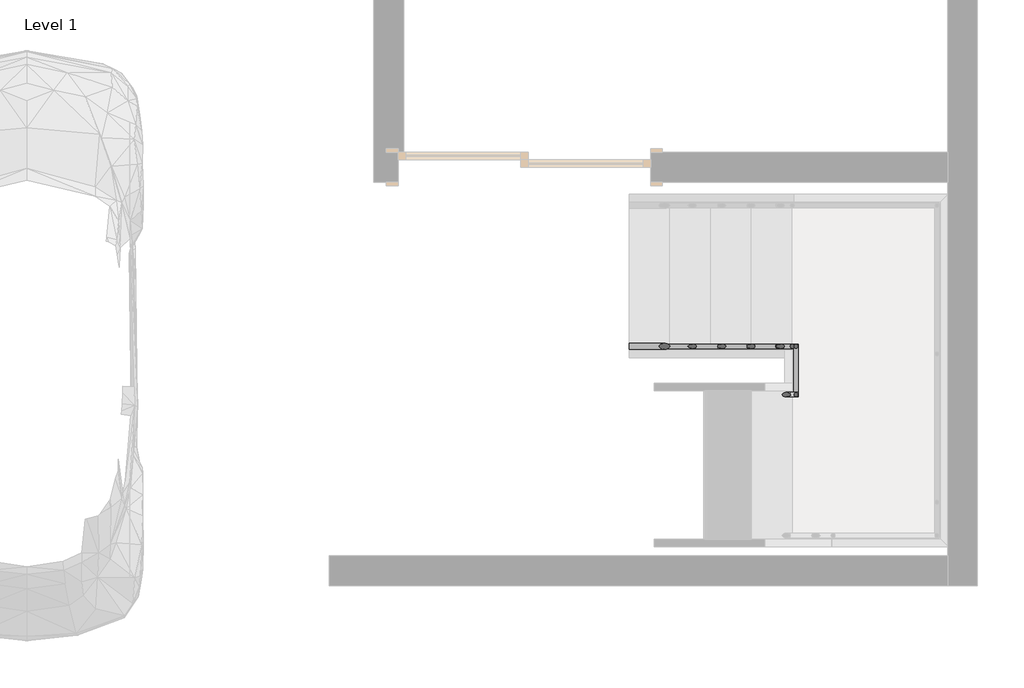
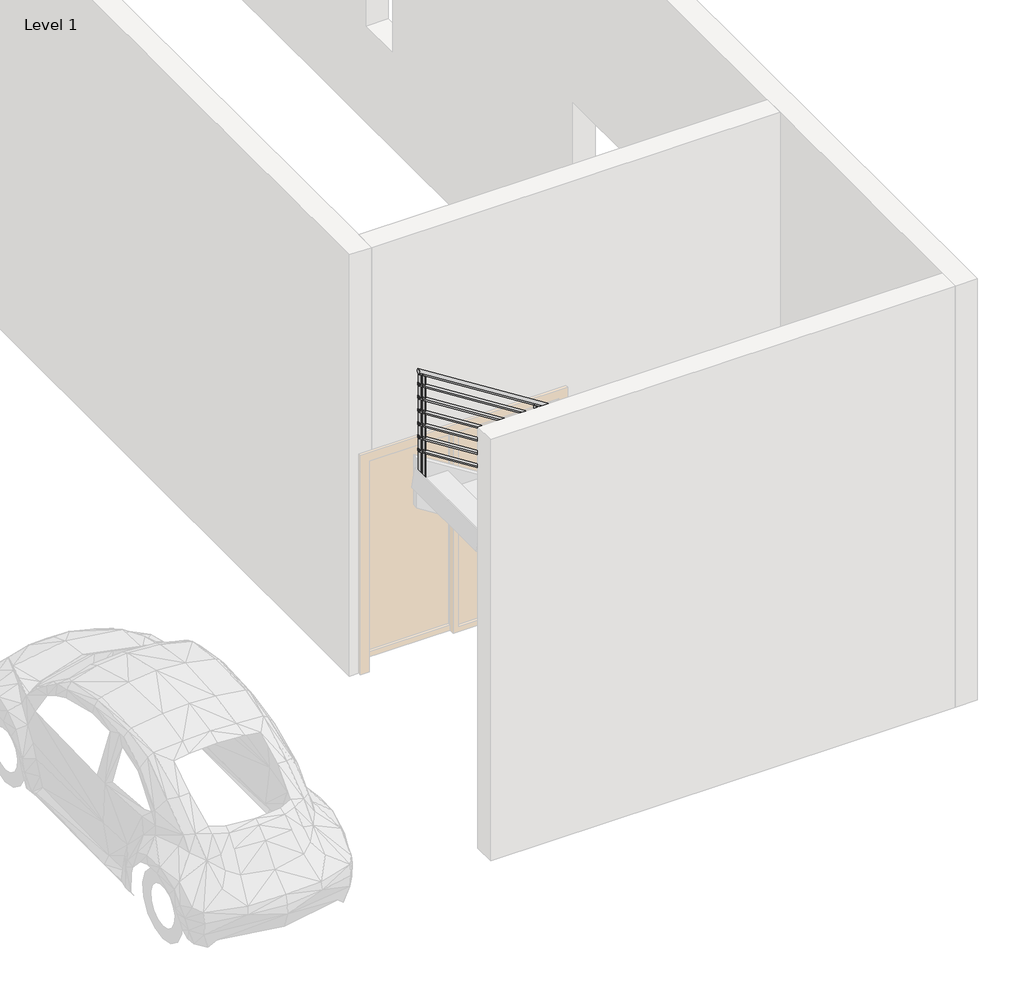
# One storey, part 2 of 4: 1 railing.
"""IFC4 building model written with IfcOpenShell, lengths in millimetres."""

from ifc_helpers import new_model, si_unit, point, frame, frame_2d, origin, place, context, project, spatial, circle_curve, ellipse_curve, trimmed, segment, composite_curve, outline, extrude, element, save
from ifc_brep_helpers import plane_surface, cylinder_surface, advanced_brep

model = new_model("IFC4")

# Units and contexts
model_context = context("Model", 3, world=origin())
ifc_project = project(units=[si_unit("LENGTHUNIT", "METRE", prefix="MILLI")], contexts=[model_context])

# Site, building, storey
site = spatial("IfcSite", under=ifc_project)
building = spatial("IfcBuilding", under=site)
storey = spatial("IfcBuildingStorey", under=building, Name="Level 1", Elevation=0.0)

# Railing
placement = place(None, origin())
element("IfcRailing", 1, ObjectType="900mm Pipe", at=placement, inside=storey, context=model_context, shape_type="SolidModel", body=[
    advanced_brep(
    [(-3791.9701746, -2535.7890637, 1050.2491997), (-3791.9701746, -2495.7890637, 1050.2491997), (-2672.7836865, -2535.7890637, 1758.0351211), (-2638.9768372, -2495.7890637, 1779.4149467)],
    [
        (0, 1, ellipse_curve(frame((-3791.9701746, -2515.7890637, 1050.2491997), z_axis=(-1.0, 0.0, 0.0), x_axis=(0.0, 0.0, -1.0)), 23.6638438, 20.0)),
        (1, 0, ellipse_curve(frame((-3791.9701746, -2515.7890637, 1050.2491997), z_axis=(-1.0, 0.0, 0.0), x_axis=(0.0, 0.0, -1.0)), 23.6638438, 20.0)),
        (2, 3, ellipse_curve(frame((-2655.8802618, -2515.7890637, 1768.7250339), z_axis=(0.5976263089853402, -0.7071067811865487, 0.3779454918484375), x_axis=(-0.5976263089853417, -0.7071067811865465, -0.3779454918484385)), 28.2842712, 20.0)),
        (3, 2, ellipse_curve(frame((-2655.8802618, -2515.7890637, 1768.7250339), z_axis=(0.5976263089853402, -0.7071067811865487, 0.3779454918484375), x_axis=(-0.5976263089853417, -0.7071067811865465, -0.3779454918484385)), 28.2842712, 20.0)),
        (0, 2),
        (3, 1),
    ],
    [
        plane_surface(frame((-3791.9701746, -2515.7890637, 1073.9130435), z_axis=(-1.0, 0.0, 0.0), x_axis=(0.0, 1.0, 0.0))),
        plane_surface(frame((-2666.5701746, -2515.7890637, 1785.6284585), z_axis=(0.5976263089853402, -0.7071067811865487, 0.3779454918484375), x_axis=(0.8017747781070186, 0.5270627453469434, -0.2817127396103774))),
        cylinder_surface(frame((-3781.2802618, -2515.7890637, 1057.0096189), z_axis=(-0.8451712313980431, 0.0, -0.5344956404098311), x_axis=(0.0, 1.0, 0.0)), 20.0),
    ],
    [
        (0, [[1, 2]]),
        (1, [[3, 4]]),
        (2, [[-1, 5, -4, 6]]),
        (2, [[-2, -6, -3, -5]]),
    ],
),
    advanced_brep(
    [(-2686.5701746, -2543.3824011, 1749.5652174), (-2646.5701746, -2509.5755518, 1749.5652174), (-2686.5701746, -2841.5890637, 1749.5652174), (-2646.5701746, -2841.5890637, 1749.5652174)],
    [
        (0, 1, ellipse_curve(frame((-2666.5701746, -2526.4789765, 1749.5652174), z_axis=(-0.5976263089853402, 0.7071067811865487, -0.3779454918484375), x_axis=(0.5976263089853421, 0.7071067811865462, 0.3779454918484387)), 28.2842712, 20.0)),
        (1, 0, ellipse_curve(frame((-2666.5701746, -2526.4789765, 1749.5652174), z_axis=(-0.5976263089853402, 0.7071067811865487, -0.3779454918484375), x_axis=(0.5976263089853421, 0.7071067811865462, 0.3779454918484387)), 28.2842712, 20.0)),
        (2, 3, ellipse_curve(frame((-2666.5701746, -2841.5890637, 1749.5652174), z_axis=(0.0, -0.7071067811865476, 0.7071067811865476), x_axis=(0.0, 0.7071067811865474, 0.7071067811865476)), 28.2842712, 20.0)),
        (3, 2, ellipse_curve(frame((-2666.5701746, -2841.5890637, 1749.5652174), z_axis=(0.0, -0.7071067811865476, 0.7071067811865476), x_axis=(0.0, 0.7071067811865474, 0.7071067811865476)), 28.2842712, 20.0)),
        (0, 2),
        (3, 1),
    ],
    [
        plane_surface(frame((-2666.5701746, -2515.7890637, 1769.5652174), z_axis=(-0.5976263089853402, 0.7071067811865487, -0.3779454918484375), x_axis=(0.8017747781070186, 0.5270627453469434, -0.2817127396103774))),
        plane_surface(frame((-2666.5701746, -2821.5890637, 1769.5652174), z_axis=(0.0, -0.7071067811865476, 0.7071067811865476), x_axis=(1.0, 0.0, 0.0))),
        cylinder_surface(frame((-2666.5701746, -2515.7890637, 1749.5652174), z_axis=(0.0, 1.0, 0.0), x_axis=(1.0, 0.0, 0.0)), 20.0),
    ],
    [
        (0, [[1, 2]]),
        (1, [[3, 4]]),
        (2, [[-1, 5, -4, 6]]),
        (2, [[-2, -6, -3, -5]]),
    ],
),
    advanced_brep(
    [(-2686.5701746, -2841.5890637, 1749.5652174), (-2646.5701746, -2841.5890637, 1749.5652174), (-2686.5701746, -2841.5890637, 1892.7355535), (-2646.5701746, -2841.5890637, 1914.7667984)],
    [
        (0, 1, ellipse_curve(frame((-2666.5701746, -2841.5890637, 1749.5652174), z_axis=(0.0, 0.7071067811865476, -0.7071067811865476), x_axis=(0.0, -0.7071067811865476, -0.7071067811865474)), 28.2842712, 20.0)),
        (1, 0, ellipse_curve(frame((-2666.5701746, -2841.5890637, 1749.5652174), z_axis=(0.0, 0.7071067811865476, -0.7071067811865476), x_axis=(0.0, -0.7071067811865476, -0.7071067811865474)), 28.2842712, 20.0)),
        (2, 3, ellipse_curve(frame((-2666.5701746, -2841.5890637, 1903.751176), z_axis=(-0.4824439654458172, 0.0, 0.8759268349610686), x_axis=(-0.8759268349610686, 0.0, -0.48244396544581725)), 22.8329573, 20.0)),
        (3, 2, ellipse_curve(frame((-2666.5701746, -2841.5890637, 1903.751176), z_axis=(-0.4824439654458172, 0.0, 0.8759268349610686), x_axis=(-0.8759268349610686, 0.0, -0.48244396544581725)), 22.8329573, 20.0)),
        (0, 2),
        (3, 1),
    ],
    [
        plane_surface(frame((-2666.5701746, -2841.5890637, 1749.5652174), z_axis=(0.0, 0.7071067811865476, -0.7071067811865476), x_axis=(1.0, 0.0, 0.0))),
        plane_surface(frame((-2666.5701746, -2841.5890637, 1903.751176), z_axis=(-0.4824439654458172, 0.0, 0.8759268349610686), x_axis=(0.8759268349610686, 0.0, 0.4824439654458172))),
        cylinder_surface(frame((-2666.5701746, -2841.5890637, 1749.5652174), z_axis=(0.0, 0.0, -1.0), x_axis=(1.0, 0.0, 0.0)), 20.0),
    ],
    [
        (0, [[1, 2]]),
        (1, [[3, 4]]),
        (2, [[-1, 5, -4, 6]]),
        (2, [[-2, -6, -3, -5]]),
    ],
),
    advanced_brep(
    [(-2666.5701746, -2821.5890637, 1903.751176), (-2666.5701746, -2861.5890637, 1903.751176), (-5716.9701746, -2821.5890637, 3832.8578953), (-5716.9701746, -2861.5890637, 3832.8578953)],
    [
        (0, 1, ellipse_curve(frame((-2666.5701746, -2841.5890637, 1903.751176), z_axis=(0.4824439654458172, 0.0, -0.8759268349610686), x_axis=(0.8759268349610686, 0.0, 0.48244396544581714)), 22.8329573, 20.0)),
        (1, 0, ellipse_curve(frame((-2666.5701746, -2841.5890637, 1903.751176), z_axis=(0.4824439654458172, 0.0, -0.8759268349610686), x_axis=(0.8759268349610686, 0.0, 0.48244396544581714)), 22.8329573, 20.0)),
        (2, 3, ellipse_curve(frame((-5716.9701746, -2841.5890637, 3832.8578953), z_axis=(-1.0, 0.0, 0.0), x_axis=(0.0, 0.0, -1.0)), 23.6638438, 20.0)),
        (3, 2, ellipse_curve(frame((-5716.9701746, -2841.5890637, 3832.8578953), z_axis=(-1.0, 0.0, 0.0), x_axis=(0.0, 0.0, -1.0)), 23.6638438, 20.0)),
        (0, 2),
        (3, 1),
    ],
    [
        plane_surface(frame((-2646.5701746, -2841.5890637, 1914.7667984), z_axis=(0.4824439654458172, 0.0, -0.8759268349610686), x_axis=(0.8759268349610686, 0.0, 0.4824439654458172))),
        plane_surface(frame((-5716.9701746, -2841.5890637, 3856.5217391), z_axis=(-1.0, 0.0, 0.0), x_axis=(0.0, -1.0, 0.0))),
        cylinder_surface(frame((-2657.2600874, -2841.5890637, 1897.8633738), z_axis=(0.8451712313980437, 0.0, -0.5344956404098302), x_axis=(0.0, -1.0, 0.0)), 20.0),
    ],
    [
        (0, [[1, 2]]),
        (1, [[3, 4]]),
        (2, [[-1, 5, -4, 6]]),
        (2, [[-2, -6, -3, -5]]),
    ],
),
    advanced_brep(
    [(-3791.9701746, -2500.7890637, 931.1651606), (-3791.9701746, -2530.7890637, 931.1651606), (-2687.6250849, -2500.7890637, 1629.5652174), (-2687.6250849, -2530.7890637, 1629.5652174), (-2651.5701746, -2500.7890637, 1629.5652174), (-2681.5701746, -2530.7890637, 1629.5652174), (-2651.5701746, -2826.5890637, 1629.5652174), (-2681.5701746, -2826.5890637, 1629.5652174)],
    [
        (0, 1, ellipse_curve(frame((-3791.9701746, -2515.7890637, 931.1651606), z_axis=(-1.0, 0.0, 0.0), x_axis=(0.0, 0.0, -1.0)), 17.7478828, 15.0)),
        (1, 0, ellipse_curve(frame((-3791.9701746, -2515.7890637, 931.1651606), z_axis=(-1.0, 0.0, 0.0), x_axis=(0.0, 0.0, -1.0)), 17.7478828, 15.0)),
        (0, 2),
        (2, 3, ellipse_curve(frame((-2687.6250849, -2515.7890637, 1629.5652174), z_axis=(-0.9605132043335072, 0.0, -0.2782344053149761), x_axis=(0.27823440531497673, 0.0, -0.960513204333507)), 15.6166515, 15.0)),
        (3, 1),
        (3, 2, ellipse_curve(frame((-2687.6250849, -2515.7890637, 1629.5652174), z_axis=(-0.9605132043335072, 0.0, -0.2782344053149761), x_axis=(0.27823440531497673, 0.0, -0.960513204333507)), 15.6166515, 15.0)),
        (2, 4),
        (4, 5, ellipse_curve(frame((-2666.5701746, -2515.7890637, 1629.5652174), z_axis=(-0.7071067811865461, 0.7071067811865488, 0.0), x_axis=(-0.7071067811865489, -0.707106781186546, 0.0)), 21.2132034, 15.0)),
        (5, 3),
        (5, 4, ellipse_curve(frame((-2666.5701746, -2515.7890637, 1629.5652174), z_axis=(-0.7071067811865461, 0.7071067811865488, 0.0), x_axis=(-0.7071067811865489, -0.707106781186546, 0.0)), 21.2132034, 15.0)),
        (6, 7, circle_curve(frame((-2666.5701746, -2826.5890637, 1629.5652174), z_axis=(0.0, -1.0, 0.0), x_axis=(-1.0, 0.0, 0.0)), 15.0)),
        (7, 6, circle_curve(frame((-2666.5701746, -2826.5890637, 1629.5652174), z_axis=(0.0, -1.0, 0.0), x_axis=(-1.0, 0.0, 0.0)), 15.0)),
        (4, 6),
        (7, 5),
    ],
    [
        plane_surface(frame((-3791.9701746, -2515.7890637, 948.9130435), z_axis=(-1.0, 0.0, 0.0), x_axis=(0.0, 1.0, 0.0))),
        cylinder_surface(frame((-3783.95274, -2515.7890637, 936.235475), z_axis=(-0.8451712313980433, 0.0, -0.534495640409831), x_axis=(0.0, -1.0, 0.0)), 15.0),
        cylinder_surface(frame((-2691.9701746, -2515.7890637, 1629.5652174), z_axis=(-1.0, 0.0, 0.0), x_axis=(0.0, -1.0, 0.0)), 15.0),
        plane_surface(frame((-2666.5701746, -2826.5890637, 1644.5652174), z_axis=(0.0, -1.0, 0.0), x_axis=(0.0, 0.0, -1.0))),
        cylinder_surface(frame((-2666.5701746, -2515.7890637, 1629.5652174), z_axis=(0.0, 1.0, 0.0), x_axis=(-1.0, 0.0, 0.0)), 15.0),
    ],
    [
        (0, [[1, 2]]),
        (1, [[-1, 3, 4, 5]]),
        (1, [[-2, -5, 6, -3]]),
        (2, [[-4, 7, 8, 9]]),
        (2, [[-6, -9, 10, -7]]),
        (3, [[11, 12]]),
        (4, [[-8, 13, -12, 14]]),
        (4, [[-10, -14, -11, -13]]),
    ],
),
    advanced_brep(
    [(-2651.5701746, -2856.5890637, 1775.1809709), (-2651.5701746, -2826.5890637, 1775.1809709), (-5716.9701746, -2856.5890637, 3713.7738563), (-5716.9701746, -2826.5890637, 3713.7738563)],
    [
        (0, 1, ellipse_curve(frame((-2651.5701746, -2841.5890637, 1775.1809709), z_axis=(1.0, 0.0, 0.0), x_axis=(0.0, 0.0, -1.0)), 17.7478828, 15.0)),
        (1, 0, ellipse_curve(frame((-2651.5701746, -2841.5890637, 1775.1809709), z_axis=(1.0, 0.0, 0.0), x_axis=(0.0, 0.0, -1.0)), 17.7478828, 15.0)),
        (2, 3, ellipse_curve(frame((-5716.9701746, -2841.5890637, 3713.7738563), z_axis=(-1.0, 0.0, 0.0), x_axis=(0.0, 0.0, -1.0)), 17.7478828, 15.0)),
        (3, 2, ellipse_curve(frame((-5716.9701746, -2841.5890637, 3713.7738563), z_axis=(-1.0, 0.0, 0.0), x_axis=(0.0, 0.0, -1.0)), 17.7478828, 15.0)),
        (0, 2),
        (3, 1),
    ],
    [
        plane_surface(frame((-2651.5701746, -2841.5890637, 1792.9288538), z_axis=(1.0, 0.0, 0.0), x_axis=(0.0, -1.0, 0.0))),
        plane_surface(frame((-5716.9701746, -2841.5890637, 3731.5217391), z_axis=(-1.0, 0.0, 0.0), x_axis=(0.0, -1.0, 0.0))),
        cylinder_surface(frame((-2659.5876092, -2841.5890637, 1780.2512853), z_axis=(0.8451712313980437, 0.0, -0.5344956404098302), x_axis=(0.0, 1.0, 0.0)), 15.0),
    ],
    [
        (0, [[1, 2]]),
        (1, [[3, 4]]),
        (2, [[-1, 5, -4, 6]]),
        (2, [[-2, -6, -3, -5]]),
    ],
),
    advanced_brep(
    [(-3791.9701746, -2500.7890637, 806.1651606), (-3791.9701746, -2530.7890637, 806.1651606), (-2687.6250849, -2500.7890637, 1504.5652174), (-2687.6250849, -2530.7890637, 1504.5652174), (-2651.5701746, -2500.7890637, 1504.5652174), (-2681.5701746, -2530.7890637, 1504.5652174), (-2651.5701746, -2826.5890637, 1504.5652174), (-2681.5701746, -2826.5890637, 1504.5652174)],
    [
        (0, 1, ellipse_curve(frame((-3791.9701746, -2515.7890637, 806.1651606), z_axis=(-1.0, 0.0, 0.0), x_axis=(0.0, 0.0, -1.0)), 17.7478828, 15.0)),
        (1, 0, ellipse_curve(frame((-3791.9701746, -2515.7890637, 806.1651606), z_axis=(-1.0, 0.0, 0.0), x_axis=(0.0, 0.0, -1.0)), 17.7478828, 15.0)),
        (0, 2),
        (2, 3, ellipse_curve(frame((-2687.6250849, -2515.7890637, 1504.5652174), z_axis=(-0.9605132043335072, 0.0, -0.2782344053149761), x_axis=(0.27823440531497673, 0.0, -0.960513204333507)), 15.6166515, 15.0)),
        (3, 1),
        (3, 2, ellipse_curve(frame((-2687.6250849, -2515.7890637, 1504.5652174), z_axis=(-0.9605132043335072, 0.0, -0.2782344053149761), x_axis=(0.27823440531497673, 0.0, -0.960513204333507)), 15.6166515, 15.0)),
        (2, 4),
        (4, 5, ellipse_curve(frame((-2666.5701746, -2515.7890637, 1504.5652174), z_axis=(-0.7071067811865461, 0.7071067811865488, 0.0), x_axis=(-0.7071067811865489, -0.707106781186546, 0.0)), 21.2132034, 15.0)),
        (5, 3),
        (5, 4, ellipse_curve(frame((-2666.5701746, -2515.7890637, 1504.5652174), z_axis=(-0.7071067811865461, 0.7071067811865488, 0.0), x_axis=(-0.7071067811865489, -0.707106781186546, 0.0)), 21.2132034, 15.0)),
        (6, 7, circle_curve(frame((-2666.5701746, -2826.5890637, 1504.5652174), z_axis=(0.0, -1.0, 0.0), x_axis=(-1.0, 0.0, 0.0)), 15.0)),
        (7, 6, circle_curve(frame((-2666.5701746, -2826.5890637, 1504.5652174), z_axis=(0.0, -1.0, 0.0), x_axis=(-1.0, 0.0, 0.0)), 15.0)),
        (4, 6),
        (7, 5),
    ],
    [
        plane_surface(frame((-3791.9701746, -2515.7890637, 823.9130435), z_axis=(-1.0, 0.0, 0.0), x_axis=(0.0, 1.0, 0.0))),
        cylinder_surface(frame((-3783.95274, -2515.7890637, 811.235475), z_axis=(-0.8451712313980433, 0.0, -0.534495640409831), x_axis=(0.0, -1.0, 0.0)), 15.0),
        cylinder_surface(frame((-2691.9701746, -2515.7890637, 1504.5652174), z_axis=(-1.0, 0.0, 0.0), x_axis=(0.0, -1.0, 0.0)), 15.0),
        plane_surface(frame((-2666.5701746, -2826.5890637, 1519.5652174), z_axis=(0.0, -1.0, 0.0), x_axis=(0.0, 0.0, -1.0))),
        cylinder_surface(frame((-2666.5701746, -2515.7890637, 1504.5652174), z_axis=(0.0, 1.0, 0.0), x_axis=(-1.0, 0.0, 0.0)), 15.0),
    ],
    [
        (0, [[1, 2]]),
        (1, [[-1, 3, 4, 5]]),
        (1, [[-2, -5, 6, -3]]),
        (2, [[-4, 7, 8, 9]]),
        (2, [[-6, -9, 10, -7]]),
        (3, [[11, 12]]),
        (4, [[-8, 13, -12, 14]]),
        (4, [[-10, -14, -11, -13]]),
    ],
),
    advanced_brep(
    [(-2651.5701746, -2856.5890637, 1650.1809709), (-2651.5701746, -2826.5890637, 1650.1809709), (-5716.9701746, -2856.5890637, 3588.7738563), (-5716.9701746, -2826.5890637, 3588.7738563)],
    [
        (0, 1, ellipse_curve(frame((-2651.5701746, -2841.5890637, 1650.1809709), z_axis=(1.0, 0.0, 0.0), x_axis=(0.0, 0.0, -1.0)), 17.7478828, 15.0)),
        (1, 0, ellipse_curve(frame((-2651.5701746, -2841.5890637, 1650.1809709), z_axis=(1.0, 0.0, 0.0), x_axis=(0.0, 0.0, -1.0)), 17.7478828, 15.0)),
        (2, 3, ellipse_curve(frame((-5716.9701746, -2841.5890637, 3588.7738563), z_axis=(-1.0, 0.0, 0.0), x_axis=(0.0, 0.0, -1.0)), 17.7478828, 15.0)),
        (3, 2, ellipse_curve(frame((-5716.9701746, -2841.5890637, 3588.7738563), z_axis=(-1.0, 0.0, 0.0), x_axis=(0.0, 0.0, -1.0)), 17.7478828, 15.0)),
        (0, 2),
        (3, 1),
    ],
    [
        plane_surface(frame((-2651.5701746, -2841.5890637, 1667.9288538), z_axis=(1.0, 0.0, 0.0), x_axis=(0.0, -1.0, 0.0))),
        plane_surface(frame((-5716.9701746, -2841.5890637, 3606.5217391), z_axis=(-1.0, 0.0, 0.0), x_axis=(0.0, -1.0, 0.0))),
        cylinder_surface(frame((-2659.5876092, -2841.5890637, 1655.2512853), z_axis=(0.8451712313980437, 0.0, -0.5344956404098302), x_axis=(0.0, 1.0, 0.0)), 15.0),
    ],
    [
        (0, [[1, 2]]),
        (1, [[3, 4]]),
        (2, [[-1, 5, -4, 6]]),
        (2, [[-2, -6, -3, -5]]),
    ],
),
    advanced_brep(
    [(-3791.9701746, -2500.7890637, 681.1651606), (-3791.9701746, -2530.7890637, 681.1651606), (-2687.6250849, -2500.7890637, 1379.5652174), (-2687.6250849, -2530.7890637, 1379.5652174), (-2651.5701746, -2500.7890637, 1379.5652174), (-2681.5701746, -2530.7890637, 1379.5652174), (-2651.5701746, -2826.5890637, 1379.5652174), (-2681.5701746, -2826.5890637, 1379.5652174)],
    [
        (0, 1, ellipse_curve(frame((-3791.9701746, -2515.7890637, 681.1651606), z_axis=(-1.0, 0.0, 0.0), x_axis=(0.0, 0.0, -1.0)), 17.7478828, 15.0)),
        (1, 0, ellipse_curve(frame((-3791.9701746, -2515.7890637, 681.1651606), z_axis=(-1.0, 0.0, 0.0), x_axis=(0.0, 0.0, -1.0)), 17.7478828, 15.0)),
        (0, 2),
        (2, 3, ellipse_curve(frame((-2687.6250849, -2515.7890637, 1379.5652174), z_axis=(-0.9605132043335072, 0.0, -0.2782344053149761), x_axis=(0.27823440531497673, 0.0, -0.960513204333507)), 15.6166515, 15.0)),
        (3, 1),
        (3, 2, ellipse_curve(frame((-2687.6250849, -2515.7890637, 1379.5652174), z_axis=(-0.9605132043335072, 0.0, -0.2782344053149761), x_axis=(0.27823440531497673, 0.0, -0.960513204333507)), 15.6166515, 15.0)),
        (2, 4),
        (4, 5, ellipse_curve(frame((-2666.5701746, -2515.7890637, 1379.5652174), z_axis=(-0.7071067811865461, 0.7071067811865488, 0.0), x_axis=(-0.7071067811865489, -0.707106781186546, 0.0)), 21.2132034, 15.0)),
        (5, 3),
        (5, 4, ellipse_curve(frame((-2666.5701746, -2515.7890637, 1379.5652174), z_axis=(-0.7071067811865461, 0.7071067811865488, 0.0), x_axis=(-0.7071067811865489, -0.707106781186546, 0.0)), 21.2132034, 15.0)),
        (6, 7, circle_curve(frame((-2666.5701746, -2826.5890637, 1379.5652174), z_axis=(0.0, -1.0, 0.0), x_axis=(-1.0, 0.0, 0.0)), 15.0)),
        (7, 6, circle_curve(frame((-2666.5701746, -2826.5890637, 1379.5652174), z_axis=(0.0, -1.0, 0.0), x_axis=(-1.0, 0.0, 0.0)), 15.0)),
        (4, 6),
        (7, 5),
    ],
    [
        plane_surface(frame((-3791.9701746, -2515.7890637, 698.9130435), z_axis=(-1.0, 0.0, 0.0), x_axis=(0.0, 1.0, 0.0))),
        cylinder_surface(frame((-3783.95274, -2515.7890637, 686.235475), z_axis=(-0.8451712313980433, 0.0, -0.534495640409831), x_axis=(0.0, -1.0, 0.0)), 15.0),
        cylinder_surface(frame((-2691.9701746, -2515.7890637, 1379.5652174), z_axis=(-1.0, 0.0, 0.0), x_axis=(0.0, -1.0, 0.0)), 15.0),
        plane_surface(frame((-2666.5701746, -2826.5890637, 1394.5652174), z_axis=(0.0, -1.0, 0.0), x_axis=(0.0, 0.0, -1.0))),
        cylinder_surface(frame((-2666.5701746, -2515.7890637, 1379.5652174), z_axis=(0.0, 1.0, 0.0), x_axis=(-1.0, 0.0, 0.0)), 15.0),
    ],
    [
        (0, [[1, 2]]),
        (1, [[-1, 3, 4, 5]]),
        (1, [[-2, -5, 6, -3]]),
        (2, [[-4, 7, 8, 9]]),
        (2, [[-6, -9, 10, -7]]),
        (3, [[11, 12]]),
        (4, [[-8, 13, -12, 14]]),
        (4, [[-10, -14, -11, -13]]),
    ],
),
    advanced_brep(
    [(-2651.5701746, -2856.5890637, 1525.1809709), (-2651.5701746, -2826.5890637, 1525.1809709), (-5716.9701746, -2856.5890637, 3463.7738563), (-5716.9701746, -2826.5890637, 3463.7738563)],
    [
        (0, 1, ellipse_curve(frame((-2651.5701746, -2841.5890637, 1525.1809709), z_axis=(1.0, 0.0, 0.0), x_axis=(0.0, 0.0, -1.0)), 17.7478828, 15.0)),
        (1, 0, ellipse_curve(frame((-2651.5701746, -2841.5890637, 1525.1809709), z_axis=(1.0, 0.0, 0.0), x_axis=(0.0, 0.0, -1.0)), 17.7478828, 15.0)),
        (2, 3, ellipse_curve(frame((-5716.9701746, -2841.5890637, 3463.7738563), z_axis=(-1.0, 0.0, 0.0), x_axis=(0.0, 0.0, -1.0)), 17.7478828, 15.0)),
        (3, 2, ellipse_curve(frame((-5716.9701746, -2841.5890637, 3463.7738563), z_axis=(-1.0, 0.0, 0.0), x_axis=(0.0, 0.0, -1.0)), 17.7478828, 15.0)),
        (0, 2),
        (3, 1),
    ],
    [
        plane_surface(frame((-2651.5701746, -2841.5890637, 1542.9288538), z_axis=(1.0, 0.0, 0.0), x_axis=(0.0, -1.0, 0.0))),
        plane_surface(frame((-5716.9701746, -2841.5890637, 3481.5217391), z_axis=(-1.0, 0.0, 0.0), x_axis=(0.0, -1.0, 0.0))),
        cylinder_surface(frame((-2659.5876092, -2841.5890637, 1530.2512853), z_axis=(0.8451712313980437, 0.0, -0.5344956404098301), x_axis=(0.0, 1.0, 0.0)), 15.0),
    ],
    [
        (0, [[1, 2]]),
        (1, [[3, 4]]),
        (2, [[-1, 5, -4, 6]]),
        (2, [[-2, -6, -3, -5]]),
    ],
),
    advanced_brep(
    [(-3791.9701746, -2500.7890637, 556.1651606), (-3791.9701746, -2530.7890637, 556.1651606), (-2687.6250849, -2500.7890637, 1254.5652174), (-2687.6250849, -2530.7890637, 1254.5652174), (-2651.5701746, -2500.7890637, 1254.5652174), (-2681.5701746, -2530.7890637, 1254.5652174), (-2651.5701746, -2826.5890637, 1254.5652174), (-2681.5701746, -2826.5890637, 1254.5652174)],
    [
        (0, 1, ellipse_curve(frame((-3791.9701746, -2515.7890637, 556.1651606), z_axis=(-1.0, 0.0, 0.0), x_axis=(0.0, 0.0, -1.0)), 17.7478828, 15.0)),
        (1, 0, ellipse_curve(frame((-3791.9701746, -2515.7890637, 556.1651606), z_axis=(-1.0, 0.0, 0.0), x_axis=(0.0, 0.0, -1.0)), 17.7478828, 15.0)),
        (0, 2),
        (2, 3, ellipse_curve(frame((-2687.6250849, -2515.7890637, 1254.5652174), z_axis=(-0.9605132043335072, 0.0, -0.2782344053149761), x_axis=(0.27823440531497673, 0.0, -0.960513204333507)), 15.6166515, 15.0)),
        (3, 1),
        (3, 2, ellipse_curve(frame((-2687.6250849, -2515.7890637, 1254.5652174), z_axis=(-0.9605132043335072, 0.0, -0.2782344053149761), x_axis=(0.27823440531497673, 0.0, -0.960513204333507)), 15.6166515, 15.0)),
        (2, 4),
        (4, 5, ellipse_curve(frame((-2666.5701746, -2515.7890637, 1254.5652174), z_axis=(-0.7071067811865461, 0.7071067811865488, 0.0), x_axis=(-0.7071067811865489, -0.707106781186546, 0.0)), 21.2132034, 15.0)),
        (5, 3),
        (5, 4, ellipse_curve(frame((-2666.5701746, -2515.7890637, 1254.5652174), z_axis=(-0.7071067811865461, 0.7071067811865488, 0.0), x_axis=(-0.7071067811865489, -0.707106781186546, 0.0)), 21.2132034, 15.0)),
        (6, 7, circle_curve(frame((-2666.5701746, -2826.5890637, 1254.5652174), z_axis=(0.0, -1.0, 0.0), x_axis=(-1.0, 0.0, 0.0)), 15.0)),
        (7, 6, circle_curve(frame((-2666.5701746, -2826.5890637, 1254.5652174), z_axis=(0.0, -1.0, 0.0), x_axis=(-1.0, 0.0, 0.0)), 15.0)),
        (4, 6),
        (7, 5),
    ],
    [
        plane_surface(frame((-3791.9701746, -2515.7890637, 573.9130435), z_axis=(-1.0, 0.0, 0.0), x_axis=(0.0, 1.0, 0.0))),
        cylinder_surface(frame((-3783.95274, -2515.7890637, 561.235475), z_axis=(-0.8451712313980433, 0.0, -0.534495640409831), x_axis=(0.0, -1.0, 0.0)), 15.0),
        cylinder_surface(frame((-2691.9701746, -2515.7890637, 1254.5652174), z_axis=(-1.0, 0.0, 0.0), x_axis=(0.0, -1.0, 0.0)), 15.0),
        plane_surface(frame((-2666.5701746, -2826.5890637, 1269.5652174), z_axis=(0.0, -1.0, 0.0), x_axis=(0.0, 0.0, -1.0))),
        cylinder_surface(frame((-2666.5701746, -2515.7890637, 1254.5652174), z_axis=(0.0, 1.0, 0.0), x_axis=(-1.0, 0.0, 0.0)), 15.0),
    ],
    [
        (0, [[1, 2]]),
        (1, [[-1, 3, 4, 5]]),
        (1, [[-2, -5, 6, -3]]),
        (2, [[-4, 7, 8, 9]]),
        (2, [[-6, -9, 10, -7]]),
        (3, [[11, 12]]),
        (4, [[-8, 13, -12, 14]]),
        (4, [[-10, -14, -11, -13]]),
    ],
),
    advanced_brep(
    [(-2651.5701746, -2856.5890637, 1400.1809709), (-2651.5701746, -2826.5890637, 1400.1809709), (-5716.9701746, -2856.5890637, 3338.7738563), (-5716.9701746, -2826.5890637, 3338.7738563)],
    [
        (0, 1, ellipse_curve(frame((-2651.5701746, -2841.5890637, 1400.1809709), z_axis=(1.0, 0.0, 0.0), x_axis=(0.0, 0.0, -1.0)), 17.7478828, 15.0)),
        (1, 0, ellipse_curve(frame((-2651.5701746, -2841.5890637, 1400.1809709), z_axis=(1.0, 0.0, 0.0), x_axis=(0.0, 0.0, -1.0)), 17.7478828, 15.0)),
        (2, 3, ellipse_curve(frame((-5716.9701746, -2841.5890637, 3338.7738563), z_axis=(-1.0, 0.0, 0.0), x_axis=(0.0, 0.0, -1.0)), 17.7478828, 15.0)),
        (3, 2, ellipse_curve(frame((-5716.9701746, -2841.5890637, 3338.7738563), z_axis=(-1.0, 0.0, 0.0), x_axis=(0.0, 0.0, -1.0)), 17.7478828, 15.0)),
        (0, 2),
        (3, 1),
    ],
    [
        plane_surface(frame((-2651.5701746, -2841.5890637, 1417.9288538), z_axis=(1.0, 0.0, 0.0), x_axis=(0.0, -1.0, 0.0))),
        plane_surface(frame((-5716.9701746, -2841.5890637, 3356.5217391), z_axis=(-1.0, 0.0, 0.0), x_axis=(0.0, -1.0, 0.0))),
        cylinder_surface(frame((-2659.5876092, -2841.5890637, 1405.2512853), z_axis=(0.8451712313980437, 0.0, -0.5344956404098302), x_axis=(0.0, 1.0, 0.0)), 15.0),
    ],
    [
        (0, [[1, 2]]),
        (1, [[3, 4]]),
        (2, [[-1, 5, -4, 6]]),
        (2, [[-2, -6, -3, -5]]),
    ],
),
    advanced_brep(
    [(-3791.9701746, -2500.7890637, 431.1651606), (-3791.9701746, -2530.7890637, 431.1651606), (-2687.6250849, -2500.7890637, 1129.5652174), (-2687.6250849, -2530.7890637, 1129.5652174), (-2651.5701746, -2500.7890637, 1129.5652174), (-2681.5701746, -2530.7890637, 1129.5652174), (-2651.5701746, -2826.5890637, 1129.5652174), (-2681.5701746, -2826.5890637, 1129.5652174)],
    [
        (0, 1, ellipse_curve(frame((-3791.9701746, -2515.7890637, 431.1651606), z_axis=(-1.0, 0.0, 0.0), x_axis=(0.0, 0.0, -1.0)), 17.7478828, 15.0)),
        (1, 0, ellipse_curve(frame((-3791.9701746, -2515.7890637, 431.1651606), z_axis=(-1.0, 0.0, 0.0), x_axis=(0.0, 0.0, -1.0)), 17.7478828, 15.0)),
        (0, 2),
        (2, 3, ellipse_curve(frame((-2687.6250849, -2515.7890637, 1129.5652174), z_axis=(-0.9605132043335072, 0.0, -0.2782344053149761), x_axis=(0.27823440531497673, 0.0, -0.960513204333507)), 15.6166515, 15.0)),
        (3, 1),
        (3, 2, ellipse_curve(frame((-2687.6250849, -2515.7890637, 1129.5652174), z_axis=(-0.9605132043335072, 0.0, -0.2782344053149761), x_axis=(0.27823440531497673, 0.0, -0.960513204333507)), 15.6166515, 15.0)),
        (2, 4),
        (4, 5, ellipse_curve(frame((-2666.5701746, -2515.7890637, 1129.5652174), z_axis=(-0.7071067811865461, 0.7071067811865488, 0.0), x_axis=(-0.7071067811865489, -0.707106781186546, 0.0)), 21.2132034, 15.0)),
        (5, 3),
        (5, 4, ellipse_curve(frame((-2666.5701746, -2515.7890637, 1129.5652174), z_axis=(-0.7071067811865461, 0.7071067811865488, 0.0), x_axis=(-0.7071067811865489, -0.707106781186546, 0.0)), 21.2132034, 15.0)),
        (6, 7, circle_curve(frame((-2666.5701746, -2826.5890637, 1129.5652174), z_axis=(0.0, -1.0, 0.0), x_axis=(-1.0, 0.0, 0.0)), 15.0)),
        (7, 6, circle_curve(frame((-2666.5701746, -2826.5890637, 1129.5652174), z_axis=(0.0, -1.0, 0.0), x_axis=(-1.0, 0.0, 0.0)), 15.0)),
        (4, 6),
        (7, 5),
    ],
    [
        plane_surface(frame((-3791.9701746, -2515.7890637, 448.9130435), z_axis=(-1.0, 0.0, 0.0), x_axis=(0.0, 1.0, 0.0))),
        cylinder_surface(frame((-3783.95274, -2515.7890637, 436.235475), z_axis=(-0.8451712313980433, 0.0, -0.534495640409831), x_axis=(0.0, -1.0, 0.0)), 15.0),
        cylinder_surface(frame((-2691.9701746, -2515.7890637, 1129.5652174), z_axis=(-1.0, 0.0, 0.0), x_axis=(0.0, -1.0, 0.0)), 15.0),
        plane_surface(frame((-2666.5701746, -2826.5890637, 1144.5652174), z_axis=(0.0, -1.0, 0.0), x_axis=(0.0, 0.0, -1.0))),
        cylinder_surface(frame((-2666.5701746, -2515.7890637, 1129.5652174), z_axis=(0.0, 1.0, 0.0), x_axis=(-1.0, 0.0, 0.0)), 15.0),
    ],
    [
        (0, [[1, 2]]),
        (1, [[-1, 3, 4, 5]]),
        (1, [[-2, -5, 6, -3]]),
        (2, [[-4, 7, 8, 9]]),
        (2, [[-6, -9, 10, -7]]),
        (3, [[11, 12]]),
        (4, [[-8, 13, -12, 14]]),
        (4, [[-10, -14, -11, -13]]),
    ],
),
    advanced_brep(
    [(-2651.5701746, -2856.5890637, 1275.1809709), (-2651.5701746, -2826.5890637, 1275.1809709), (-5716.9701746, -2856.5890637, 3213.7738563), (-5716.9701746, -2826.5890637, 3213.7738563)],
    [
        (0, 1, ellipse_curve(frame((-2651.5701746, -2841.5890637, 1275.1809709), z_axis=(1.0, 0.0, 0.0), x_axis=(0.0, 0.0, -1.0)), 17.7478828, 15.0)),
        (1, 0, ellipse_curve(frame((-2651.5701746, -2841.5890637, 1275.1809709), z_axis=(1.0, 0.0, 0.0), x_axis=(0.0, 0.0, -1.0)), 17.7478828, 15.0)),
        (2, 3, ellipse_curve(frame((-5716.9701746, -2841.5890637, 3213.7738563), z_axis=(-1.0, 0.0, 0.0), x_axis=(0.0, 0.0, -1.0)), 17.7478828, 15.0)),
        (3, 2, ellipse_curve(frame((-5716.9701746, -2841.5890637, 3213.7738563), z_axis=(-1.0, 0.0, 0.0), x_axis=(0.0, 0.0, -1.0)), 17.7478828, 15.0)),
        (0, 2),
        (3, 1),
    ],
    [
        plane_surface(frame((-2651.5701746, -2841.5890637, 1292.9288538), z_axis=(1.0, 0.0, 0.0), x_axis=(0.0, -1.0, 0.0))),
        plane_surface(frame((-5716.9701746, -2841.5890637, 3231.5217391), z_axis=(-1.0, 0.0, 0.0), x_axis=(0.0, -1.0, 0.0))),
        cylinder_surface(frame((-2659.5876092, -2841.5890637, 1280.2512853), z_axis=(0.8451712313980437, 0.0, -0.5344956404098302), x_axis=(0.0, 1.0, 0.0)), 15.0),
    ],
    [
        (0, [[1, 2]]),
        (1, [[3, 4]]),
        (2, [[-1, 5, -4, 6]]),
        (2, [[-2, -6, -3, -5]]),
    ],
),
    advanced_brep(
    [(-3791.9701746, -2500.7890637, 306.1651606), (-3791.9701746, -2530.7890637, 306.1651606), (-2687.6250849, -2500.7890637, 1004.5652174), (-2687.6250849, -2530.7890637, 1004.5652174), (-2651.5701746, -2500.7890637, 1004.5652174), (-2681.5701746, -2530.7890637, 1004.5652174), (-2651.5701746, -2826.5890637, 1004.5652174), (-2681.5701746, -2826.5890637, 1004.5652174)],
    [
        (0, 1, ellipse_curve(frame((-3791.9701746, -2515.7890637, 306.1651606), z_axis=(-1.0, 0.0, 0.0), x_axis=(0.0, 0.0, -1.0)), 17.7478828, 15.0)),
        (1, 0, ellipse_curve(frame((-3791.9701746, -2515.7890637, 306.1651606), z_axis=(-1.0, 0.0, 0.0), x_axis=(0.0, 0.0, -1.0)), 17.7478828, 15.0)),
        (0, 2),
        (2, 3, ellipse_curve(frame((-2687.6250849, -2515.7890637, 1004.5652174), z_axis=(-0.9605132043335072, 0.0, -0.2782344053149761), x_axis=(0.27823440531497673, 0.0, -0.960513204333507)), 15.6166515, 15.0)),
        (3, 1),
        (3, 2, ellipse_curve(frame((-2687.6250849, -2515.7890637, 1004.5652174), z_axis=(-0.9605132043335072, 0.0, -0.2782344053149761), x_axis=(0.27823440531497673, 0.0, -0.960513204333507)), 15.6166515, 15.0)),
        (2, 4),
        (4, 5, ellipse_curve(frame((-2666.5701746, -2515.7890637, 1004.5652174), z_axis=(-0.7071067811865461, 0.7071067811865488, 0.0), x_axis=(-0.7071067811865489, -0.707106781186546, 0.0)), 21.2132034, 15.0)),
        (5, 3),
        (5, 4, ellipse_curve(frame((-2666.5701746, -2515.7890637, 1004.5652174), z_axis=(-0.7071067811865461, 0.7071067811865488, 0.0), x_axis=(-0.7071067811865489, -0.707106781186546, 0.0)), 21.2132034, 15.0)),
        (6, 7, circle_curve(frame((-2666.5701746, -2826.5890637, 1004.5652174), z_axis=(0.0, -1.0, 0.0), x_axis=(-1.0, 0.0, 0.0)), 15.0)),
        (7, 6, circle_curve(frame((-2666.5701746, -2826.5890637, 1004.5652174), z_axis=(0.0, -1.0, 0.0), x_axis=(-1.0, 0.0, 0.0)), 15.0)),
        (4, 6),
        (7, 5),
    ],
    [
        plane_surface(frame((-3791.9701746, -2515.7890637, 323.9130435), z_axis=(-1.0, 0.0, 0.0), x_axis=(0.0, 1.0, 0.0))),
        cylinder_surface(frame((-3783.95274, -2515.7890637, 311.235475), z_axis=(-0.8451712313980433, 0.0, -0.534495640409831), x_axis=(0.0, -1.0, 0.0)), 15.0),
        cylinder_surface(frame((-2691.9701746, -2515.7890637, 1004.5652174), z_axis=(-1.0, 0.0, 0.0), x_axis=(0.0, -1.0, 0.0)), 15.0),
        plane_surface(frame((-2666.5701746, -2826.5890637, 1019.5652174), z_axis=(0.0, -1.0, 0.0), x_axis=(0.0, 0.0, -1.0))),
        cylinder_surface(frame((-2666.5701746, -2515.7890637, 1004.5652174), z_axis=(0.0, 1.0, 0.0), x_axis=(-1.0, 0.0, 0.0)), 15.0),
    ],
    [
        (0, [[1, 2]]),
        (1, [[-1, 3, 4, 5]]),
        (1, [[-2, -5, 6, -3]]),
        (2, [[-4, 7, 8, 9]]),
        (2, [[-6, -9, 10, -7]]),
        (3, [[11, 12]]),
        (4, [[-8, 13, -12, 14]]),
        (4, [[-10, -14, -11, -13]]),
    ],
),
    advanced_brep(
    [(-2651.5701746, -2856.5890637, 1150.1809709), (-2651.5701746, -2826.5890637, 1150.1809709), (-5716.9701746, -2856.5890637, 3088.7738563), (-5716.9701746, -2826.5890637, 3088.7738563)],
    [
        (0, 1, ellipse_curve(frame((-2651.5701746, -2841.5890637, 1150.1809709), z_axis=(1.0, 0.0, 0.0), x_axis=(0.0, 0.0, -1.0)), 17.7478828, 15.0)),
        (1, 0, ellipse_curve(frame((-2651.5701746, -2841.5890637, 1150.1809709), z_axis=(1.0, 0.0, 0.0), x_axis=(0.0, 0.0, -1.0)), 17.7478828, 15.0)),
        (2, 3, ellipse_curve(frame((-5716.9701746, -2841.5890637, 3088.7738563), z_axis=(-1.0, 0.0, 0.0), x_axis=(0.0, 0.0, -1.0)), 17.7478828, 15.0)),
        (3, 2, ellipse_curve(frame((-5716.9701746, -2841.5890637, 3088.7738563), z_axis=(-1.0, 0.0, 0.0), x_axis=(0.0, 0.0, -1.0)), 17.7478828, 15.0)),
        (0, 2),
        (3, 1),
    ],
    [
        plane_surface(frame((-2651.5701746, -2841.5890637, 1167.9288538), z_axis=(1.0, 0.0, 0.0), x_axis=(0.0, -1.0, 0.0))),
        plane_surface(frame((-5716.9701746, -2841.5890637, 3106.5217391), z_axis=(-1.0, 0.0, 0.0), x_axis=(0.0, -1.0, 0.0))),
        cylinder_surface(frame((-2659.5876092, -2841.5890637, 1155.2512853), z_axis=(0.8451712313980437, 0.0, -0.5344956404098302), x_axis=(0.0, 1.0, 0.0)), 15.0),
    ],
    [
        (0, [[1, 2]]),
        (1, [[3, 4]]),
        (2, [[-1, 5, -4, 6]]),
        (2, [[-2, -6, -3, -5]]),
    ],
),
    advanced_brep(
    [(-5666.5701746, -2829.0890637, 3777.3205338), (-5666.5701746, -2829.0890637, 2782.6086957), (-5666.5701746, -2854.0890637, 2782.6086957), (-5666.5701746, -2854.0890637, 3777.3205338)],
    [
        (0, 1),
        (1, 2, circle_curve(frame((-5666.5701746, -2841.5890637, 2782.6086957), z_axis=(0.0, 0.0, 1.0), x_axis=(0.0, -1.0, 0.0)), 12.5)),
        (2, 3),
        (3, 0, ellipse_curve(frame((-5666.5701746, -2841.5890637, 3777.3205338), z_axis=(-0.5344956404098286, 0.0, -0.8451712313980447), x_axis=(-0.8451712313980447, 0.0, 0.5344956404098286)), 14.7899024, 12.5)),
        (0, 3, ellipse_curve(frame((-5666.5701746, -2841.5890637, 3777.3205338), z_axis=(-0.5344956404098286, 0.0, -0.8451712313980447), x_axis=(-0.8451712313980447, 0.0, 0.5344956404098286)), 14.7899024, 12.5)),
        (2, 1, circle_curve(frame((-5666.5701746, -2841.5890637, 2782.6086957), z_axis=(0.0, 0.0, 1.0), x_axis=(0.0, -1.0, 0.0)), 12.5)),
    ],
    [
        cylinder_surface(frame((-5666.5701746, -2841.5890637, 2682.6086957), z_axis=(0.0, 0.0, 1.0), x_axis=(0.0, -1.0, 0.0)), 12.5),
        plane_surface(frame((-5691.5701746, -2866.5890637, 3793.1308104), z_axis=(0.5344956404098286, 0.0, 0.8451712313980447), x_axis=(0.0, 1.0, 0.0))),
        plane_surface(frame((-5641.5701746, -2866.5890637, 2782.6086957), z_axis=(0.0, 0.0, -1.0), x_axis=(0.0, 1.0, 0.0))),
    ],
    [
        (0, [[1, 2, 3, 4]]),
        (0, [[-1, 5, -3, 6]]),
        (1, [[-4, -5]]),
        (2, [[-2, -6]]),
    ],
),
    advanced_brep(
    [(-4666.5701746, -2829.0890637, 3144.9094666), (-4666.5701746, -2829.0890637, 2260.8695652), (-4666.5701746, -2854.0890637, 2260.8695652), (-4666.5701746, -2854.0890637, 3144.9094666)],
    [
        (0, 1),
        (1, 2, circle_curve(frame((-4666.5701746, -2841.5890637, 2260.8695652), z_axis=(0.0, 0.0, 1.0), x_axis=(0.0, -1.0, 0.0)), 12.5)),
        (2, 3),
        (3, 0, ellipse_curve(frame((-4666.5701746, -2841.5890637, 3144.9094666), z_axis=(-0.5344956404098286, 0.0, -0.8451712313980447), x_axis=(-0.8451712313980447, 0.0, 0.5344956404098286)), 14.7899024, 12.5)),
        (0, 3, ellipse_curve(frame((-4666.5701746, -2841.5890637, 3144.9094666), z_axis=(-0.5344956404098286, 0.0, -0.8451712313980447), x_axis=(-0.8451712313980447, 0.0, 0.5344956404098286)), 14.7899024, 12.5)),
        (2, 1, circle_curve(frame((-4666.5701746, -2841.5890637, 2260.8695652), z_axis=(0.0, 0.0, 1.0), x_axis=(0.0, -1.0, 0.0)), 12.5)),
    ],
    [
        cylinder_surface(frame((-4666.5701746, -2841.5890637, 2160.8695652), z_axis=(0.0, 0.0, 1.0), x_axis=(0.0, -1.0, 0.0)), 12.5),
        plane_surface(frame((-4691.5701746, -2866.5890637, 3160.7197432), z_axis=(0.5344956404098286, 0.0, 0.8451712313980447), x_axis=(0.0, 1.0, 0.0))),
        plane_surface(frame((-4641.5701746, -2866.5890637, 2260.8695652), z_axis=(0.0, 0.0, -1.0), x_axis=(0.0, 1.0, 0.0))),
    ],
    [
        (0, [[1, 2, 3, 4]]),
        (0, [[-1, 5, -3, 6]]),
        (1, [[-4, -5]]),
        (2, [[-2, -6]]),
    ],
),
    advanced_brep(
    [(-3666.5701746, -2829.0890637, 2512.4983994), (-3666.5701746, -2829.0890637, 1565.2173913), (-3666.5701746, -2854.0890637, 1565.2173913), (-3666.5701746, -2854.0890637, 2512.4983994)],
    [
        (0, 1),
        (1, 2, circle_curve(frame((-3666.5701746, -2841.5890637, 1565.2173913), z_axis=(0.0, 0.0, 1.0), x_axis=(0.0, -1.0, 0.0)), 12.5)),
        (2, 3),
        (3, 0, ellipse_curve(frame((-3666.5701746, -2841.5890637, 2512.4983994), z_axis=(-0.5344956404098302, 0.0, -0.8451712313980437), x_axis=(-0.8451712313980437, 0.0, 0.53449564040983)), 14.7899024, 12.5)),
        (0, 3, ellipse_curve(frame((-3666.5701746, -2841.5890637, 2512.4983994), z_axis=(-0.5344956404098302, 0.0, -0.8451712313980437), x_axis=(-0.8451712313980437, 0.0, 0.53449564040983)), 14.7899024, 12.5)),
        (2, 1, circle_curve(frame((-3666.5701746, -2841.5890637, 1565.2173913), z_axis=(0.0, 0.0, 1.0), x_axis=(0.0, -1.0, 0.0)), 12.5)),
    ],
    [
        cylinder_surface(frame((-3666.5701746, -2841.5890637, 1465.2173913), z_axis=(0.0, 0.0, 1.0), x_axis=(0.0, -1.0, 0.0)), 12.5),
        plane_surface(frame((-3691.5701746, -2866.5890637, 2528.308676), z_axis=(0.5344956404098302, 0.0, 0.8451712313980437), x_axis=(0.0, 1.0, 0.0))),
        plane_surface(frame((-3641.5701746, -2866.5890637, 1565.2173913), z_axis=(0.0, 0.0, -1.0), x_axis=(0.0, 1.0, 0.0))),
    ],
    [
        (0, [[1, 2, 3, 4]]),
        (0, [[-1, 5, -3, 6]]),
        (1, [[-4, -5]]),
        (2, [[-2, -6]]),
    ],
),
    advanced_brep(
    [(-2791.9701746, -2528.2890637, 1658.9964231), (-2791.9701746, -2528.2890637, 695.6521739), (-2791.9701746, -2503.2890637, 695.6521739), (-2791.9701746, -2503.2890637, 1658.9964231)],
    [
        (0, 1),
        (1, 2, circle_curve(frame((-2791.9701746, -2515.7890637, 695.6521739), z_axis=(0.0, 0.0, 1.0), x_axis=(0.0, 1.0, 0.0)), 12.5)),
        (2, 3),
        (3, 0, ellipse_curve(frame((-2791.9701746, -2515.7890637, 1658.9964231), z_axis=(0.5344956404098302, 0.0, -0.8451712313980437), x_axis=(0.8451712313980437, 0.0, 0.53449564040983)), 14.7899024, 12.5)),
        (0, 3, ellipse_curve(frame((-2791.9701746, -2515.7890637, 1658.9964231), z_axis=(0.5344956404098302, 0.0, -0.8451712313980437), x_axis=(0.8451712313980437, 0.0, 0.53449564040983)), 14.7899024, 12.5)),
        (2, 1, circle_curve(frame((-2791.9701746, -2515.7890637, 695.6521739), z_axis=(0.0, 0.0, 1.0), x_axis=(0.0, 1.0, 0.0)), 12.5)),
    ],
    [
        cylinder_surface(frame((-2791.9701746, -2515.7890637, 595.6521739), z_axis=(0.0, 0.0, 1.0), x_axis=(0.0, 1.0, 0.0)), 12.5),
        plane_surface(frame((-2766.9701746, -2490.7890637, 1674.8066998), z_axis=(-0.5344956404098302, 0.0, 0.8451712313980437), x_axis=(0.0, -1.0, 0.0))),
        plane_surface(frame((-2816.9701746, -2490.7890637, 695.6521739), z_axis=(0.0, 0.0, -1.0), x_axis=(0.0, -1.0, 0.0))),
    ],
    [
        (0, [[1, 2, 3, 4]]),
        (0, [[-1, 5, -3, 6]]),
        (1, [[-4, -5]]),
        (2, [[-2, -6]]),
    ],
),
    extrude(outline(composite_curve([segment(trimmed(circle_curve(frame_2d((-2666.5701746, -2841.5890637)), 12.5), [point((-2666.5701746, -2854.0890637))], [point((-2666.5701746, -2829.0890637))], False, "CARTESIAN"), True, "CONTINUOUS"), segment(trimmed(circle_curve(frame_2d((-2666.5701746, -2841.5890637)), 12.5), [point((-2666.5701746, -2829.0890637))], [point((-2666.5701746, -2854.0890637))], False, "CARTESIAN"), True, "CONTINUOUS")], self_intersect=False)), frame((0.0, 0.0, 869.5652174), z_axis=(0.0, 0.0, 1.0), x_axis=(1.0, 0.0, 0.0)), (0.0, 0.0, 1.0), 860.0),
    advanced_brep(
    [(-2666.5701746, -2528.2890637, 1738.3007709), (-2666.5701746, -2528.2890637, 869.5652174), (-2666.5701746, -2503.2890637, 869.5652174), (-2666.5701746, -2503.2890637, 1738.3007709)],
    [
        (0, 1),
        (1, 2, circle_curve(frame((-2666.5701746, -2515.7890637, 869.5652174), z_axis=(0.0, 0.0, 1.0), x_axis=(0.0, 1.0, 0.0)), 12.5)),
        (2, 3),
        (3, 0, ellipse_curve(frame((-2666.5701746, -2515.7890637, 1738.3007709), z_axis=(0.5344956404098286, 0.0, -0.8451712313980447), x_axis=(0.8451712313980447, 0.0, 0.5344956404098286)), 14.7899024, 12.5)),
        (0, 3, ellipse_curve(frame((-2666.5701746, -2515.7890637, 1738.3007709), z_axis=(0.5344956404098286, 0.0, -0.8451712313980447), x_axis=(0.8451712313980447, 0.0, 0.5344956404098286)), 14.7899024, 12.5)),
        (2, 1, circle_curve(frame((-2666.5701746, -2515.7890637, 869.5652174), z_axis=(0.0, 0.0, 1.0), x_axis=(0.0, 1.0, 0.0)), 12.5)),
    ],
    [
        cylinder_surface(frame((-2666.5701746, -2515.7890637, 769.5652174), z_axis=(0.0, 0.0, 1.0), x_axis=(0.0, 1.0, 0.0)), 12.5),
        plane_surface(frame((-2641.5701746, -2490.7890637, 1754.1110476), z_axis=(-0.5344956404098286, 0.0, 0.8451712313980447), x_axis=(0.0, -1.0, 0.0))),
        plane_surface(frame((-2691.5701746, -2490.7890637, 869.5652174), z_axis=(0.0, 0.0, -1.0), x_axis=(0.0, -1.0, 0.0))),
    ],
    [
        (0, [[1, 2, 3, 4]]),
        (0, [[-1, 5, -3, 6]]),
        (1, [[-4, -5]]),
        (2, [[-2, -6]]),
    ],
),
    advanced_brep(
    [(-2691.9701746, -2528.2890637, 1722.2375298), (-2691.9701746, -2528.2890637, 869.5652174), (-2691.9701746, -2503.2890637, 869.5652174), (-2691.9701746, -2503.2890637, 1722.2375298)],
    [
        (0, 1),
        (1, 2, circle_curve(frame((-2691.9701746, -2515.7890637, 869.5652174), z_axis=(0.0, 0.0, 1.0), x_axis=(0.0, 1.0, 0.0)), 12.5)),
        (2, 3),
        (3, 0, ellipse_curve(frame((-2691.9701746, -2515.7890637, 1722.2375298), z_axis=(0.5344956404098286, 0.0, -0.8451712313980447), x_axis=(0.8451712313980447, 0.0, 0.5344956404098286)), 14.7899024, 12.5)),
        (0, 3, ellipse_curve(frame((-2691.9701746, -2515.7890637, 1722.2375298), z_axis=(0.5344956404098286, 0.0, -0.8451712313980447), x_axis=(0.8451712313980447, 0.0, 0.5344956404098286)), 14.7899024, 12.5)),
        (2, 1, circle_curve(frame((-2691.9701746, -2515.7890637, 869.5652174), z_axis=(0.0, 0.0, 1.0), x_axis=(0.0, 1.0, 0.0)), 12.5)),
    ],
    [
        cylinder_surface(frame((-2691.9701746, -2515.7890637, 769.5652174), z_axis=(0.0, 0.0, 1.0), x_axis=(0.0, 1.0, 0.0)), 12.5),
        plane_surface(frame((-2666.9701746, -2490.7890637, 1738.0478065), z_axis=(-0.5344956404098286, 0.0, 0.8451712313980447), x_axis=(0.0, -1.0, 0.0))),
        plane_surface(frame((-2716.9701746, -2490.7890637, 869.5652174), z_axis=(0.0, 0.0, -1.0), x_axis=(0.0, -1.0, 0.0))),
    ],
    [
        (0, [[1, 2, 3, 4]]),
        (0, [[-1, 5, -3, 6]]),
        (1, [[-4, -5]]),
        (2, [[-2, -6]]),
    ],
),
    advanced_brep(
    [(-5704.4701746, -2829.0890637, 3801.2889132), (-5704.4701746, -2829.0890637, 2782.6086957), (-5704.4701746, -2854.0890637, 2782.6086957), (-5704.4701746, -2854.0890637, 3801.2889132)],
    [
        (0, 1),
        (1, 2, circle_curve(frame((-5704.4701746, -2841.5890637, 2782.6086957), z_axis=(0.0, 0.0, 1.0), x_axis=(0.0, -1.0, 0.0)), 12.5)),
        (2, 3),
        (3, 0, ellipse_curve(frame((-5704.4701746, -2841.5890637, 3801.2889132), z_axis=(-0.5344956404098302, 0.0, -0.8451712313980437), x_axis=(-0.8451712313980437, 0.0, 0.53449564040983)), 14.7899024, 12.5)),
        (0, 3, ellipse_curve(frame((-5704.4701746, -2841.5890637, 3801.2889132), z_axis=(-0.5344956404098302, 0.0, -0.8451712313980437), x_axis=(-0.8451712313980437, 0.0, 0.53449564040983)), 14.7899024, 12.5)),
        (2, 1, circle_curve(frame((-5704.4701746, -2841.5890637, 2782.6086957), z_axis=(0.0, 0.0, 1.0), x_axis=(0.0, -1.0, 0.0)), 12.5)),
    ],
    [
        cylinder_surface(frame((-5704.4701746, -2841.5890637, 2682.6086957), z_axis=(0.0, 0.0, 1.0), x_axis=(0.0, -1.0, 0.0)), 12.5),
        plane_surface(frame((-5729.4701746, -2866.5890637, 3817.0991899), z_axis=(0.5344956404098302, 0.0, 0.8451712313980437), x_axis=(0.0, 1.0, 0.0))),
        plane_surface(frame((-5679.4701746, -2866.5890637, 2782.6086957), z_axis=(0.0, 0.0, -1.0), x_axis=(0.0, 1.0, 0.0))),
    ],
    [
        (0, [[1, 2, 3, 4]]),
        (0, [[-1, 5, -3, 6]]),
        (1, [[-4, -5]]),
        (2, [[-2, -6]]),
    ],
),
    advanced_brep(
    [(-3779.4701746, -2528.2890637, 1034.4904942), (-3779.4701746, -2528.2890637, 173.9130435), (-3779.4701746, -2503.2890637, 173.9130435), (-3779.4701746, -2503.2890637, 1034.4904942)],
    [
        (0, 1),
        (1, 2, circle_curve(frame((-3779.4701746, -2515.7890637, 173.9130435), z_axis=(0.0, 0.0, 1.0), x_axis=(0.0, 1.0, 0.0)), 12.5)),
        (2, 3),
        (3, 0, ellipse_curve(frame((-3779.4701746, -2515.7890637, 1034.4904942), z_axis=(0.5344956404098302, 0.0, -0.8451712313980437), x_axis=(0.8451712313980437, 0.0, 0.53449564040983)), 14.7899024, 12.5)),
        (0, 3, ellipse_curve(frame((-3779.4701746, -2515.7890637, 1034.4904942), z_axis=(0.5344956404098302, 0.0, -0.8451712313980437), x_axis=(0.8451712313980437, 0.0, 0.53449564040983)), 14.7899024, 12.5)),
        (2, 1, circle_curve(frame((-3779.4701746, -2515.7890637, 173.9130435), z_axis=(0.0, 0.0, 1.0), x_axis=(0.0, 1.0, 0.0)), 12.5)),
    ],
    [
        cylinder_surface(frame((-3779.4701746, -2515.7890637, 73.9130435), z_axis=(0.0, 0.0, 1.0), x_axis=(0.0, 1.0, 0.0)), 12.5),
        plane_surface(frame((-3754.4701746, -2490.7890637, 1050.3007709), z_axis=(-0.5344956404098302, 0.0, 0.8451712313980437), x_axis=(0.0, -1.0, 0.0))),
        plane_surface(frame((-3804.4701746, -2490.7890637, 173.9130435), z_axis=(0.0, 0.0, -1.0), x_axis=(0.0, -1.0, 0.0))),
    ],
    [
        (0, [[1, 2, 3, 4]]),
        (0, [[-1, 5, -3, 6]]),
        (1, [[-4, -5]]),
        (2, [[-2, -6]]),
    ],
),
])

save(model, "model.ifc")

# Revit data of these elements
# Type "900mm Pipe"
#   built-in parameter 1008612 = 0.019685 (stored number, unit not read)
#   built-in parameter 1008611 = 0.0984252 (stored number, unit not read)
#   built-in parameter 1008609 = 6.56168 (stored number, unit not read)
#   built-in parameter 1008604 = 0.19685 (stored number, unit not read)
#   built-in parameter 1008603 = 0.164042 (stored number, unit not read)
#   Railing Height = 2' - 11.43307"
#   built-in parameter 1008630 = 2
#   built-in parameter 1008610 = 2
#   built-in parameter 1008605 = 1
#   built-in parameter 1008618 = M_Baluster - Round : 25mm
# Element 1 (IfcRailing, "900mm Pipe")
#   Phase Created = New Construction
